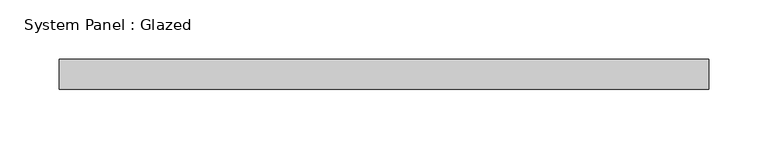
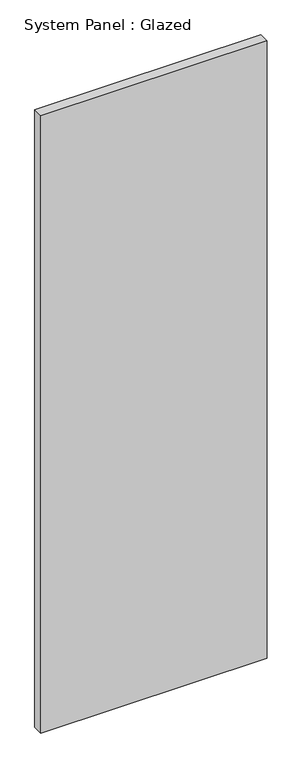
"""IFC4 building model written with IfcOpenShell, lengths in millimetres: plate geometry, System Panel : Glazed."""

from ifc_helpers import new_model, si_unit, origin, origin_with_axes, place, context, project, spatial, polyline, outline, extrude, source, transform, mapped, element, save


def system_panel_glazed_62cbeebf(model_context):
    return source(origin(), model_context, "Body", "SweptSolid", [
        extrude(outline(polyline([(274.1083333, 19.05), (-274.1083333, 19.05), (-274.1083333, 44.45), (274.1083333, 44.45), (274.1083333, 19.05)])), origin_with_axes(), (0.0, 0.0, 1.0), 1581.0857893),
    ])


if __name__ == "__main__":
    model = new_model("IFC4")
    model_context = context("Model", 3, world=origin())
    ifc_project = project(units=[si_unit("LENGTHUNIT", "METRE", prefix="MILLI")], contexts=[model_context])
    site = spatial("IfcSite", under=ifc_project)
    building = spatial("IfcBuilding", under=site)
    placement = place(None, origin())
    system_panel_glazed_shape = system_panel_glazed_62cbeebf(model_context)
    element("IfcPlate", 1, ObjectType="System Panel : Glazed", at=placement, inside=building, context=model_context, shape_type="MappedRepresentation", body=[
        mapped(system_panel_glazed_shape, transform((0.0, 0.0, 0.0), x_axis=(1.0, 0.0, 0.0), y_axis=(0.0, 1.0, 0.0), z_axis=(0.0, 0.0, 1.0))),
    ])
    save(model, "model.ifc")

# Revit data of these elements
# Type "System Panel : Glazed"
#   Construction Type Id = "GSP4R"
#   Analytic Construction = "1/8 in Pilkington single glazing"
#   Visual Light Transmittance = 0.9
#   Solar Heat Gain Coefficient = 0.86
#   Heat Transfer Coefficient (U) = 1.18115 BTU/(h·ft²·°F)
# Element 1 (IfcPlate, "System Panel : Glazed")
#   Materials on its faces: "Glass"
# Materials
#   "Glass": class "Glass", colour RGB 0 128 192, transparency 0.75, Description = "Soda Lime Glass", Cost = 0
